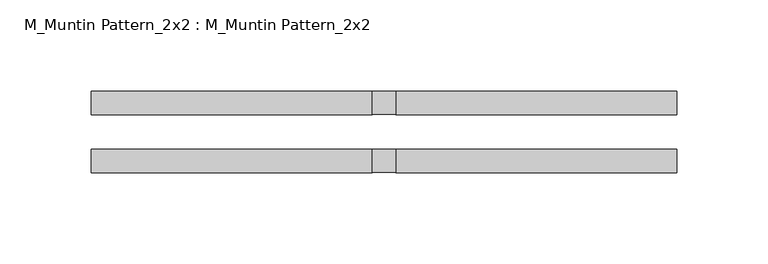
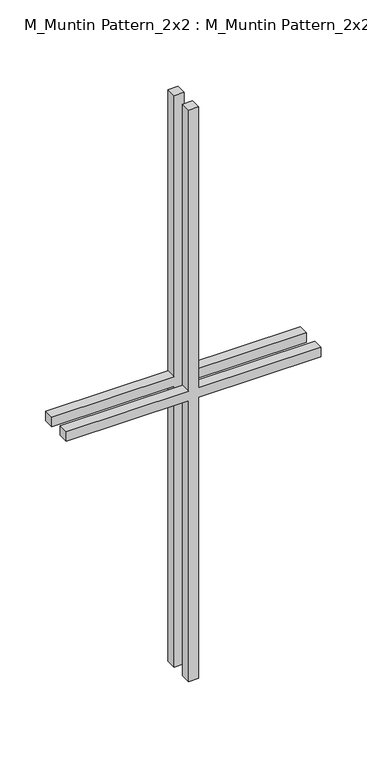
"""IFC4 building model written with IfcOpenShell, lengths in millimetres: proxy geometry, M_Muntin Pattern_2x2 : M_Muntin Pattern_2x2."""

from ifc_helpers import new_model, si_unit, frame, origin, place, context, project, spatial, polyline, outline, extrude, source, transform, mapped, element, save


def m_muntin_pattern_2x2_m_muntin_pattern_2x2_55460d9e(model_context):
    return source(origin(), model_context, "Body", "SweptSolid", [
        extrude(outline(polyline([(386.5, -6.35), (386.5, -160.3375), (373.8, -160.3375), (373.8, -6.35), (0.0, -6.35), (0.0, 6.35), (373.8, 6.35), (373.8, 160.3375), (386.5, 160.3375), (386.5, 6.35), (760.3, 6.35), (760.3, -6.35), (386.5, -6.35)])), frame((0.0, 9.525, 0.0), z_axis=(0.0, 1.0, 0.0), x_axis=(0.0, 0.0, 1.0)), (0.0, 0.0, 1.0), 12.7),
        extrude(outline(polyline([(386.5, -6.35), (386.5, -160.3375), (373.8, -160.3375), (373.8, -6.35), (0.0, -6.35), (0.0, 6.35), (373.8, 6.35), (373.8, 160.3375), (386.5, 160.3375), (386.5, 6.35), (760.3, 6.35), (760.3, -6.35), (386.5, -6.35)])), frame((0.0, -22.225, 0.0), z_axis=(0.0, 1.0, 0.0), x_axis=(0.0, 0.0, 1.0)), (0.0, 0.0, 1.0), 12.7),
    ])


if __name__ == "__main__":
    model = new_model("IFC4")
    model_context = context("Model", 3, world=origin())
    ifc_project = project(units=[si_unit("LENGTHUNIT", "METRE", prefix="MILLI")], contexts=[model_context])
    site = spatial("IfcSite", under=ifc_project)
    building = spatial("IfcBuilding", under=site)
    placement = place(None, origin())
    m_muntin_pattern_2x2_m_muntin_pattern_2x2_shape = m_muntin_pattern_2x2_m_muntin_pattern_2x2_55460d9e(model_context)
    element("IfcBuildingElementProxy", 1, Name="M_Muntin Pattern_2x2 : M_Muntin Pattern_2x2", ObjectType="M_Muntin Pattern_2x2 : M_Muntin Pattern_2x2", at=placement, inside=building, context=model_context, shape_type="MappedRepresentation", body=[
        mapped(m_muntin_pattern_2x2_m_muntin_pattern_2x2_shape, transform((0.0, 0.0, 0.0), x_axis=(1.0, 0.0, 0.0), y_axis=(0.0, 1.0, 0.0), z_axis=(0.0, 0.0, 1.0))),
    ])
    save(model, "model.ifc")

# Revit data of these elements
# Type "M_Muntin Pattern_2x2 : M_Muntin Pattern_2x2"
#   Width [instance default] = 3' - 11.24409"
#   Thickness = 0' - 0 1/2"
#   Height [instance default] = 3' - 11.24409"
#   Distance = 0' - 0 3/4"
#   Interior Material [instance default] = none
#   Exterior Material [instance default] = none
#   Default Elevation = 0
# Element 1 (IfcBuildingElementProxy, "M_Muntin Pattern_2x2 : M_Muntin Pattern_2x2")
#   Width = 1' - 0 5/8"
#   Height = 2' - 5.93307"
#   Interior Material = Wood - Stained
#   Exterior Material = Clad - White
#   Materials on its faces: "Clad - White", "Wood - Stained"
# Materials
#   "Clad - White": class "Wood", colour RGB 242 242 238, transparency 0, Cost = 0
#   "Wood - Stained": class "Wood", colour RGB 224 178 126, transparency 0, Cost = 0
